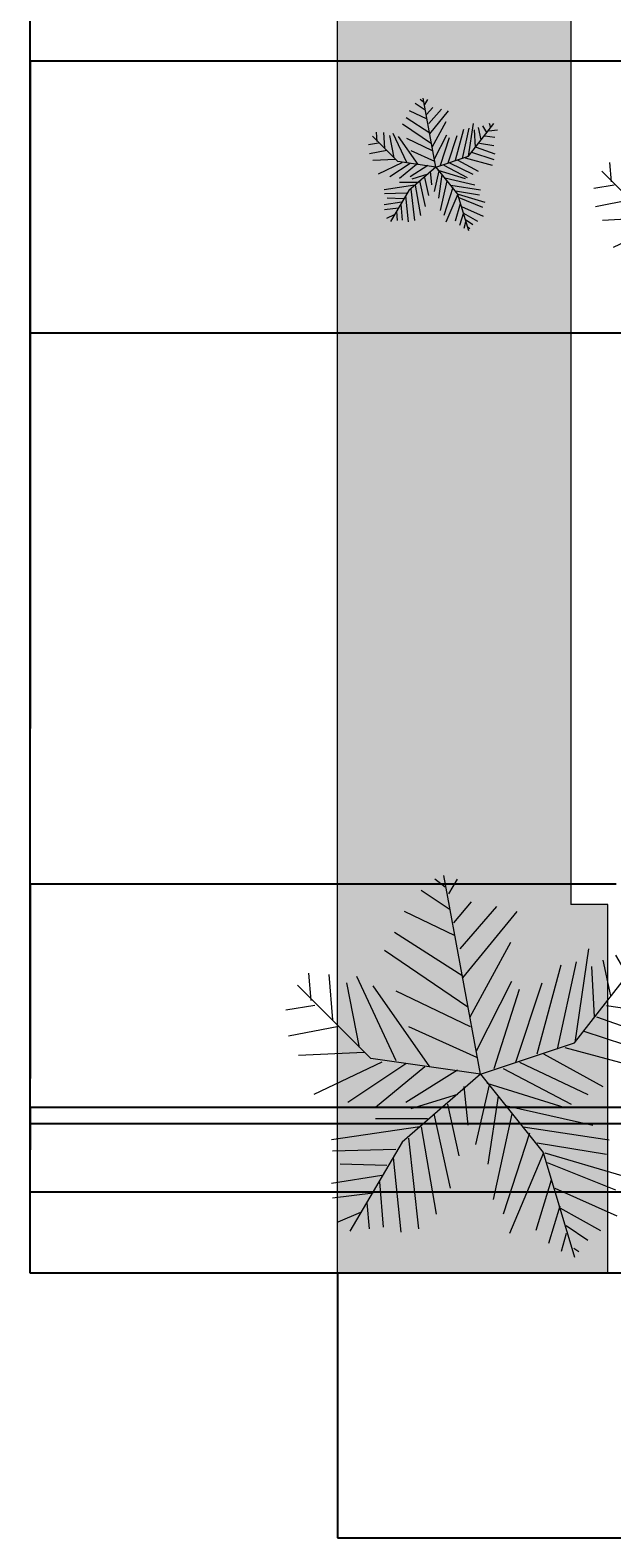
# Model space of a CAD drawing. Units: millimetres. Extents: x -229 to 16545, y -10488 to 4272.
# Tile 1 of 29: x -229 to 1930, y -10230 to -4633. Entities that reach past the tile are written whole.
import ezdxf

# ---------------------------------------------------------------- set-up
doc = ezdxf.new("R2010")
doc.units = ezdxf.units.MM
for name, color, linetype, lineweight in [('A-ANNO-DIMS', 2, 'Continuous', 18), ('L-PLNT-BEDS', 82, 'Continuous', 18), ('L-PLNT-TREE', 80, 'Continuous', 18)]:
    doc.layers.add(name, color=color, linetype=linetype, lineweight=lineweight)
doc.layers.add('L-PLNT-PATT', color=116, linetype='Continuous', lineweight=13, true_color=0x136734)
doc.styles.get("Standard").update_dxf_attribs({"font": 'arial.ttf'})
doc.dimstyles.get("Standard").update_dxf_attribs({"dimtxt": 0.18, "dimasz": 0.18, "dimexe": 0.18, "dimexo": 0.0625, "dimgap": 0.09, "dimtad": 0, "dimtih": 1, "dimtoh": 1, "dimdec": 4, "dimzin": 0, "dimdsep": 46, "dimtxsty": 'Standard', "dimcen": 0.09, "dimadec": 0, "dimazin": 0, "dimtfac": 1, "dimtdec": 4, "dimtofl": 0, "dimtmove": 0, "dimatfit": 3, "dimfxl": 1, "dimtolj": 1, "dimtzin": 0, "dimarcsym": 0})

# ---------------------------------------------------------------- blocks, each defined once
blk = doc.blocks.new('*U18')
for p, q in [((0, 0), (-10.5, 57)), ((-8.736999999999625, 47.13799999999969), (-17.06899999999996, 52.71100000000001)), ((-10.18600000000015, 53.63999999999987), (-13.08399999999983, 55.96199999999976)), ((-9.098999999999705, 51.7819999999997), (-6.563000000000101, 55.96199999999976)), ((-7.65000000000009, 43.42299999999977), (-2.577999999999974, 49.45999999999981)), ((-5.838999999999941, 35.99199999999973), (4.666999999999916, 48.06699999999977)), ((-7.28800000000001, 39.70699999999965), (-21.77800000000025, 46.67299999999977)), ((-5.114000000000032, 27.63199999999983), (10.46300000000019, 46.67299999999977)), ((-5.114000000000032, 28.09699999999975), (-24.67599999999993, 40.63599999999996)), ((-3.665000000000418, 19.27299999999968), (-27.57400000000007, 35.52699999999982)), ((-2.940999999999803, 16.48599999999987), (8.652000000000044, 37.84999999999991)), ((27, 9), (48, 36)), ((27.12699999999995, 9.05600000000004), (31.11200000000008, 35.99199999999973)), ((44.15300000000025, 36.45599999999991), (45.23900000000003, 32.74099999999999)), ((16.25900000000001, 5.804999999999836), (23.14199999999983, 31.34799999999973)), ((22.05499999999984, 7.197999999999865), (27.48900000000003, 32.27699999999982)), ((31.83600000000024, 30.88299999999981), (32.56100000000015, 16.48599999999987)), ((35.09600000000001, 32.74099999999999), (37.26999999999998, 22.52399999999989)), ((38.71900000000005, 34.13399999999979), (41.97899999999981, 28.56099999999992)), ((43.79100000000017, 29.95399999999995), (51.03600000000006, 30.88299999999981)), ((-48.58500000000003, 21.13099999999986), (-49.30899999999974, 29.02600000000007)), ((-43.51299999999992, 28.56099999999992), (-42.42699999999968, 15.55799999999976)), ((-38.44199999999955, 26.23899999999981), (-34.81899999999996, 7.662999999999783)), ((-35.54399999999987, 28.09699999999975), (-24.31399999999985, 3.946999999999661)), ((-1.128999999999905, 6.733999999999923), (9.014000000000124, 26.70399999999995)), ((10.10100000000011, 3.482999999999719), (17.70800000000008, 26.23899999999981)), ((-31.5, 4.5), (-52.5, 25.5)), ((-14.5329999999999, 2.089999999999918), (-30.83399999999983, 25.30999999999995)), ((-24.31399999999985, 23.91699999999969), (-2.940999999999803, 13.69999999999982)), ((3.942000000000007, 1.625), (11.1869999999999, 24.38099999999986)), ((40.52999999999975, 25.77499999999986), (48.86200000000008, 24.846)), ((-47.49800000000004, 19.73699999999962), (-55.83000000000038, 18.34399999999982)), ((36.18300000000045, 19.73699999999962), (48.13699999999972, 17.87999999999988)), ((-40.61500000000023, 13.69999999999982), (-55.10500000000002, 10.91299999999978)), ((-20.69099999999981, 13.69999999999982), (-1.128999999999905, 4.875999999999976)), ((33.28499999999986, 16.48599999999987), (48.86200000000008, 10.91299999999978)), ((0, 0), (27, 9)), ((29.66199999999981, 12.30699999999979), (48.13699999999972, 6.268999999999778)), ((-33.37000000000035, 6.268999999999778), (-52.20699999999988, 5.339999999999918)), ((0, 0), (-31.5, 4.5)), ((18.06999999999971, 5.804999999999836), (35.09600000000001, -3.483000000000174)), ((24.22899999999982, 7.662999999999783), (46.6880000000001, 1.625)), ((-28.29899999999998, 3.482999999999719), (-47.86000000000012, -5.805000000000063)), ((-21.41600000000017, 3.017999999999801), (-38.07899999999973, -8.128000000000384)), ((-15.98199999999951, 2.089999999999918), (-30.11000000000013, -9.521000000000186)), ((0, 0), (-22.5, -19.5)), ((-6.563000000000101, 1.161000000000058), (-21.41600000000017, -8.128000000000384)), ((0, 0), (18, -22.5)), ((6.478000000000065, 1.625), (26.03999999999996, -8.592000000000326)), ((11.1869999999999, 3.482999999999719), (30.74900000000025, -5.805000000000063)), ((-4.751999999999952, -3.483000000000174), (-3.665000000000418, -14.62900000000013)), ((2.493000000000392, -3.019000000000005), (-1.490999999999985, -20.20200000000023)), ((1.769000000000232, -2.555000000000063), (24.22899999999982, -9.521000000000186)), ((-6.563000000000101, -5.805000000000063), (-19.96699999999964, -9.985000000000127)), ((-9.460999999999785, -8.592000000000326), (-6.201000000000021, -23.4530000000002)), ((5.028999999999996, -6.270000000000209), (2.131000000000312, -25.77500000000009)), ((-15.2569999999996, -12.77200000000016), (-30.11000000000013, -12.77200000000016)), ((-13.44599999999991, -11.37800000000038), (-8.736999999999625, -32.74100000000021)), ((9.014000000000124, -11.37800000000038), (3.579999999999927, -35.99200000000019)), ((7.564999999999599, -9.056000000000267), (32.19800000000032, -14.62900000000013)), ((-17.43100000000004, -15.09400000000005), (-42.78899999999976, -18.80899999999997)), ((-17.06899999999996, -15.09400000000005), (-12.721, -40.17200000000025)), ((14.08499999999958, -16.95100000000025), (6.478000000000065, -40.17200000000025)), ((12.27399999999988, -15.09400000000005), (36.9069999999997, -18.80899999999997)), ((-24.31399999999985, -21.59600000000023), (-42.42699999999968, -22.06000000000017)), ((-22.5, -19.5), (-37.5, -45)), ((-20.69099999999981, -18.34500000000003), (-17.79300000000012, -44.35200000000032)), ((16.25900000000001, -19.73800000000028), (36.18300000000045, -22.98900000000003)), ((-26.8489999999997, -26.24000000000001), (-40.25300000000015, -25.77500000000009)), ((-25.03800000000001, -23.91800000000035), (-22.86500000000024, -45.28100000000017)), ((18.06999999999971, -22.52400000000012), (8.289000000000215, -45.74500000000012)), ((18, -22.5), (27, -52.5)), ((18.43300000000045, -22.52400000000012), (40.52999999999975, -29.02600000000007)), ((19.1569999999997, -25.31100000000015), (38.71900000000005, -33.20600000000013)), ((-28.29899999999998, -29.02600000000007), (-42.78899999999976, -31.34800000000018)), ((-30.83399999999983, -34.13499999999999), (-42.42699999999968, -35.52800000000025)), ((-29.02300000000014, -30.88400000000002), (-27.93600000000015, -43.88700000000016)), ((20.24400000000014, -30.4190000000001), (15.89699999999993, -44.81600000000026)), ((21.33100000000013, -32.74100000000021), (39.08100000000013, -40.63600000000019)), ((-32.64600000000019, -36.92100000000005), (-31.92099999999982, -44.35200000000032)), ((22.77999999999975, -37.85000000000014), (19.51900000000023, -48.53200000000015)), ((22.77999999999975, -38.31400000000008), (34.37199999999985, -44.81600000000026)), ((-34.45699999999988, -39.70800000000031), (-40.97800000000006, -42.49400000000014)), ((24.59100000000035, -45.74500000000012), (23.14199999999983, -50.85400000000004)), ((24.59100000000035, -43.42300000000022), (30.74900000000025, -47.60300000000029)), ((26.76400000000012, -49.92500000000018), (28.21300000000019, -50.85400000000004))]:
    blk.add_line(p, q)
blk = doc.blocks.new('*D46')
at = {"layer": 'A-ANNO-DIMS', "color": 0, "lineweight": -2, "transparency": 16777216}
for p, q in [((911.9897460000004, 2251.727948000001), (-228.8374730000015, 2251.727948000001)), ((-228.6574730000015, 2251.547948000002), (-228.6574730000002, -3498.090148862212)), ((-228.657472999999, -9248.092052000004), (-228.6574730000002, -3498.453955137792)), ((911.9897460000004, -9248.272052000004), (-228.837472999999, -9248.272052000004))]:
    blk.add_line(p, q, dxfattribs=at)
at = {"layer": 'A-ANNO-DIMS', "color": 0, "transparency": 16777216}
for points in [[(-228.6874730000015, 2251.547948000002), (-228.6274730000015, 2251.547948000002), (-228.6574730000015, 2251.727948000001)], [(-228.687472999999, -9248.092052000004), (-228.6274729999989, -9248.092052000004), (-228.657472999999, -9248.272052000004)]]:
    blk.add_solid(points, dxfattribs=at)
at = {"layer": 'Defpoints', "color": 0, "transparency": 16777216}
for p in [(912.0522460000003, 2251.727948000001), (-228.657472999999, -9248.272052000004), (912.0522460000003, -9248.272052000004)]:
    blk.add_point(p, dxfattribs=at)
at = {"layer": 'A-ANNO-DIMS', "color": 0, "transparency": 16777216, "insert": (-228.6574730000012, -3498.272052), "char_height": 0.18, "attachment_point": 5}
blk.add_mtext('\\A1;11500', dxfattribs=at)
blk = doc.blocks.new('*D47')
at = {"layer": 'A-ANNO-DIMS', "color": 0, "lineweight": -2, "transparency": 16777216}
for p, q in [((912.052246, -9248.334552), (912.0522459999999, -10230.221103)), ((15679.60703, -9248.334552), (15679.60703, -10230.221103)), ((912.2322459999997, -10230.041103), (8295.409228723058, -10230.041103)), ((15679.42703, -10230.041103), (8296.250047276942, -10230.041103))]:
    blk.add_line(p, q, dxfattribs=at)
at = {"layer": 'A-ANNO-DIMS', "color": 0, "transparency": 16777216}
for points in [[(912.2322459999997, -10230.011103), (912.2322459999997, -10230.071103), (912.0522459999999, -10230.041103)], [(15679.42703, -10230.011103), (15679.42703, -10230.071103), (15679.60703, -10230.041103)]]:
    blk.add_solid(points, dxfattribs=at)
at = {"layer": 'Defpoints', "color": 0, "transparency": 16777216}
for p in [(912.052246, -9248.272052), (15679.60703, -9248.272052), (15679.60703, -10230.041103)]:
    blk.add_point(p, dxfattribs=at)
at = {"layer": 'A-ANNO-DIMS', "color": 0, "transparency": 16777216, "insert": (8295.829637999997, -10230.041103), "char_height": 0.18, "attachment_point": 5}
blk.add_mtext('\\A1;14768', dxfattribs=at)
blk = doc.blocks.new('*D62')
at = {"layer": 'A-ANNO-DIMS', "color": 0, "lineweight": -2, "transparency": 16777216}
for p, q in [((5745.870529000002, -4748.272052000002), (-228.8374730000013, -4748.272052000003)), ((-228.6574730000007, -4748.452052000003), (-228.6574730000002, -6998.090148862215)), ((-228.6574729999998, -9248.092052000005), (-228.6574730000002, -6998.453955137795)), ((5745.870529000002, -9248.272052000004), (-228.8374730000003, -9248.272052000006))]:
    blk.add_line(p, q, dxfattribs=at)
at = {"layer": 'A-ANNO-DIMS', "color": 0, "transparency": 16777216}
for points in [[(-228.6874730000008, -4748.452052000003), (-228.6274730000008, -4748.452052000003), (-228.6574730000007, -4748.272052000003)], [(-228.6874729999997, -9248.092052000005), (-228.6274729999997, -9248.092052000005), (-228.6574729999998, -9248.272052000006)]]:
    blk.add_solid(points, dxfattribs=at)
at = {"layer": 'Defpoints', "color": 0, "transparency": 16777216}
for p in [(5745.933029000002, -4748.272052000002), (-228.6574729999998, -9248.272052000006), (5745.933029000002, -9248.272052000004)]:
    blk.add_point(p, dxfattribs=at)
at = {"layer": 'A-ANNO-DIMS', "color": 0, "transparency": 16777216, "insert": (-228.6574730000022, -6998.272052000003), "char_height": 0.18, "attachment_point": 5}
blk.add_mtext('\\A1;4500', dxfattribs=at)
blk = doc.blocks.new('*D92')
at = {"layer": 'A-ANNO-DIMS', "color": 0, "lineweight": -2, "transparency": 16777216}
for p, q in [((1945.870529000001, -7803.015189000004), (-228.8374730000004, -7803.015189000004)), ((-228.6574730000004, -7803.195189000004), (-228.6574730000002, -8525.461655970674)), ((-228.6574730000001, -9248.092052000004), (-228.6574730000002, -8525.825585029335)), ((2015.870529000001, -9248.272052000004), (-228.8374729999999, -9248.272052000004))]:
    blk.add_line(p, q, dxfattribs=at)
at = {"layer": 'A-ANNO-DIMS', "color": 0, "transparency": 16777216}
for points in [[(-228.6874730000004, -7803.195189000004), (-228.6274730000004, -7803.195189000004), (-228.6574730000004, -7803.015189000004)], [(-228.6874730000001, -9248.092052000004), (-228.6274730000001, -9248.092052000004), (-228.6574730000001, -9248.272052000004)]]:
    blk.add_solid(points, dxfattribs=at)
at = {"layer": 'Defpoints', "color": 0, "transparency": 16777216}
for p in [(1945.933029000001, -7803.015189000004), (-228.6574730000001, -9248.272052000004), (2015.933029000001, -9248.272052000004)]:
    blk.add_point(p, dxfattribs=at)
at = {"layer": 'A-ANNO-DIMS', "color": 0, "transparency": 16777216, "insert": (-228.6574730000026, -8525.643620500003), "char_height": 0.18, "attachment_point": 5}
blk.add_mtext('\\A1;1445.3', dxfattribs=at)
blk = doc.blocks.new('*D96')
at = {"layer": 'A-ANNO-DIMS', "color": 0, "lineweight": -2, "transparency": 16777216}
for p, q in [((4033.528927000001, -5757.644295000002), (-228.8374730000011, -5757.644295000003)), ((-228.6574730000006, -5757.824295000003), (-228.6574730000002, -7225.597539470673)), ((-228.6574729999999, -8693.734713000003), (-228.6574730000002, -7225.961468529336)), ((4027.243185000002, -8693.914713000004), (-228.837473, -8693.914713000004))]:
    blk.add_line(p, q, dxfattribs=at)
at = {"layer": 'A-ANNO-DIMS', "color": 0, "transparency": 16777216}
for points in [[(-228.6874730000005, -5757.824295000003), (-228.6274730000005, -5757.824295000003), (-228.6574730000006, -5757.644295000003)], [(-228.6874729999999, -8693.734713000003), (-228.6274729999999, -8693.734713000003), (-228.6574729999999, -8693.914713000004)]]:
    blk.add_solid(points, dxfattribs=at)
at = {"layer": 'Defpoints', "color": 0, "transparency": 16777216}
for p in [(4033.591427000001, -5757.644295000002), (-228.6574729999999, -8693.914713000004), (4027.305685000001, -8693.914713000004)]:
    blk.add_point(p, dxfattribs=at)
at = {"layer": 'A-ANNO-DIMS', "color": 0, "transparency": 16777216, "insert": (-228.6574730000022, -7225.779504000001), "char_height": 0.18, "attachment_point": 5}
blk.add_mtext('\\A1;2936', dxfattribs=at)
blk = doc.blocks.new('*D98')
at = {"layer": 'A-ANNO-DIMS', "color": 0, "lineweight": -2, "transparency": 16777216}
for p, q in [((5975.870529000001, -8632.301380000004), (-228.8374730000005, -8632.301380000006)), ((-228.6574730000003, -8632.481380000007), (-228.6574730000002, -8789.345922470675)), ((-228.6574730000002, -8946.574394000005), (-228.6574730000002, -8789.709851529336)), ((5975.870529000001, -8946.754394000001), (-228.8374730000004, -8946.754394000007))]:
    blk.add_line(p, q, dxfattribs=at)
at = {"layer": 'A-ANNO-DIMS', "color": 0, "transparency": 16777216}
for points in [[(-228.6874730000003, -8632.481380000007), (-228.6274730000003, -8632.481380000007), (-228.6574730000003, -8632.301380000006)], [(-228.6874730000002, -8946.574394000005), (-228.6274730000002, -8946.574394000005), (-228.6574730000002, -8946.754394000007)]]:
    blk.add_solid(points, dxfattribs=at)
at = {"layer": 'Defpoints', "color": 0, "transparency": 16777216}
for p in [(-228.6574730000003, -8632.301380000006), (5975.933029000001, -8632.301380000004), (5975.933029000001, -8946.754394000001)]:
    blk.add_point(p, dxfattribs=at)
at = {"layer": 'A-ANNO-DIMS', "color": 0, "transparency": 16777216, "insert": (-228.6574730000027, -8789.527887000004), "char_height": 0.18, "attachment_point": 5}
blk.add_mtext('\\A1;314.45', dxfattribs=at)

msp = doc.modelspace()

# ---------------------------------------------------------------- hatches: boundary and pattern name
at = {"layer": 'L-PLNT-PATT'}
h = msp.add_hatch(dxfattribs=at)
h.set_pattern_fill('GRASS', color=256)
h.set_pattern_definition([(90, (-8141.222001159148, -13125.50409224634), (-17.96051224, 17.96051224), [4.7625, -31.15852448]), (45, (-8141.222001159148, -13125.50409224634), (-17.96051224213831, 17.96051224213831), [4.7625, -20.6375]), (135, (-8141.222001159148, -13125.50409224634), (-17.96051224213831, -17.9605122421383), [4.7625, -20.6375])])
h.paths.add_polyline_path([(1778.330648821284, 2251.727948476911), (912.0522459164059, 2251.727948476912), (912.0522459164021, -9248.272051523087), (1778.330648821284, -9248.272051523087), (1914.943192458922, -9248.272051523087), (1914.943192458922, -7879.257903321944), (1778.330648821284, -7879.257903321944)])
h = msp.add_hatch(dxfattribs=at)
h.set_pattern_fill('GRASS', color=256, scale=5.9)
h.set_pattern_definition([(90, (-8141.222001159148, -13125.50409224634), (-105.967022216, 105.967022216), [28.09875, -183.835294432]), (45, (-8141.222001159148, -13125.50409224634), (-105.967022228616, 105.967022228616), [28.09875, -121.76125]), (135, (-8141.222001159148, -13125.50409224634), (-105.967022228616, -105.967022228616), [28.09875, -121.76125])])
h.paths.add_polyline_path([(1778.330648821284, 2251.727948476911), (912.0522459164059, 2251.727948476911), (912.052245916402, -9248.272051523087), (1778.330648821284, -9248.272051523087), (1914.943192458922, -9248.272051523087), (1914.943192458922, -7879.257903321944), (1778.330648821284, -7879.257903321944)])

# ---------------------------------------------------------------- linework, layer by layer
at = {"layer": 'L-PLNT-BEDS', "transparency": 33554554}
for p, q in [((912.0522459164021, -9248.272051523087), (912.0522459164059, 2251.727948476911)), ((1778.330648821284, -9248.272051523087), (912.0522459164021, -9248.272051523087))]:
    msp.add_line(p, q, dxfattribs=at)
at = {"layer": 'L-PLNT-BEDS', "transparency": 33554569}
msp.add_line((1778.330648821284, 2251.727948476911), (1778.330648821284, -7879.257903321944), dxfattribs=at)
at = {"layer": 'L-PLNT-BEDS', "transparency": 33554572}
for p, q in [((1914.943192458922, -7879.257903321944), (1778.330648821284, -7879.257903321944)), ((1914.943192458922, -9248.272051523087), (1914.943192458922, -7879.257903321944)), ((1778.330648821284, -9248.272051523087), (1914.943192458922, -9248.272051523087))]:
    msp.add_line(p, q, dxfattribs=at)

# ---------------------------------------------------------------- block references
at = {"layer": 'L-PLNT-TREE'}
for p, xscale, yscale, zscale in [((1277.093975217413, -5141.443832352766), 4.481031954380777, 4.481031954380777, 4.481031954380777), ((2369.423958503968, -5387.731228287581), 9.061891725250485, 9.061891725250485, 9.061891725250485), ((1442.982306165615, -8509.019337727086), 12.94000768461256, 12.94000768461256, 12.94000768461256)]:
    msp.add_blockref('*U18', p, dxfattribs=dict(at, xscale=xscale, yscale=yscale, zscale=zscale))

# ---------------------------------------------------------------- dimensions: what is measured, and where the dimension line sits
at = {"layer": 'A-ANNO-DIMS'}
for base, p1, p2, override, picture, middle in [((-228.657472999999, -9248.272052000004), (912.052246, 2251.727948), (912.052246, -9248.272052), {"dimdec": 0, "dimlfac": 1, "dimrnd": 0, "dimzin": 0, "dimdsep": 46, "dimlunit": 2}, '*D46', (-228.6574730000012, -3498.272052)), ((-228.6574729999998, -9248.272052000006), (5745.933028999999, -4748.272051999999), (5745.933028999999, -9248.272052), {"dimdec": 0, "dimlfac": 1, "dimrnd": 0, "dimzin": 0, "dimdsep": 46, "dimlunit": 2}, '*D62', (-228.6574730000022, -6998.272052000003)), ((-228.6574729999999, -8693.914713000004), (4033.591427, -5757.644295), (4027.305684999999, -8693.914713), {"dimdec": 0, "dimlfac": 1, "dimrnd": 0, "dimzin": 0, "dimdsep": 46, "dimlunit": 2}, '*D96', (-228.6574730000022, -7225.779504000001)), ((-228.6574730000001, -9248.272052000004), (1945.933029, -7803.015188999999), (2015.933029, -9248.272052), {"dimdec": 1, "dimlfac": 1, "dimrnd": 0, "dimzin": 0, "dimdsep": 46, "dimlunit": 2}, '*D92', (-228.6574730000026, -8525.643620500003)), ((-228.6574730000003, -8632.301380000006), (5975.933029, -8946.754394), (5975.933029, -8632.30138), {"dimdec": 2, "dimlfac": 1, "dimrnd": 0, "dimzin": 0, "dimdsep": 46, "dimlunit": 2}, '*D98', (-228.6574730000027, -8789.527887000004))]:
    dim = msp.add_linear_dim(base=base, p1=p1, p2=p2, angle=90, dimstyle='Standard', override=override, dxfattribs=at)
    dim.commit()
    dim.dimension.update_dxf_attribs({"geometry": picture, "text_midpoint": middle})
dim = msp.add_linear_dim(base=(15679.60703, -10230.041103), p1=(912.052246, -9248.272052), p2=(15679.60703, -9248.272052), dimstyle='Standard', override={"dimdec": 0, "dimlfac": 1, "dimrnd": 0, "dimzin": 0, "dimdsep": 46, "dimlunit": 2}, dxfattribs=at)
dim.commit()
dim.dimension.update_dxf_attribs({"geometry": '*D47', "text_midpoint": (8295.829637999997, -10230.041103)})

doc.saveas('drawing.dxf')
